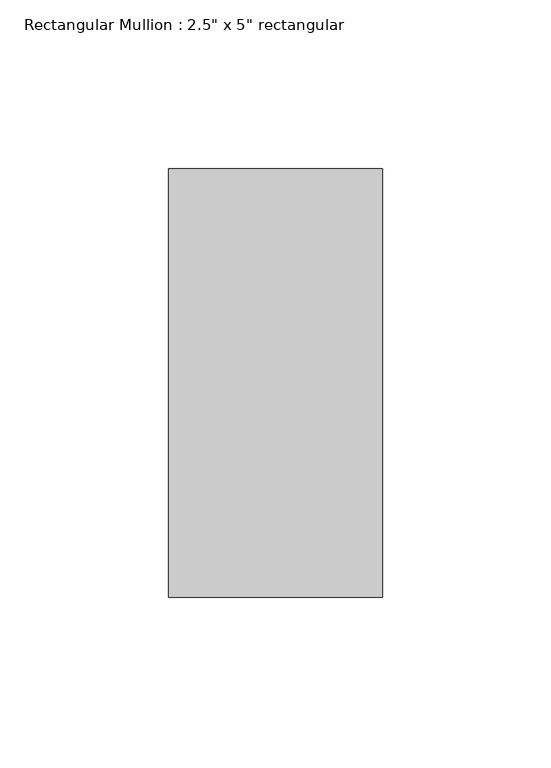
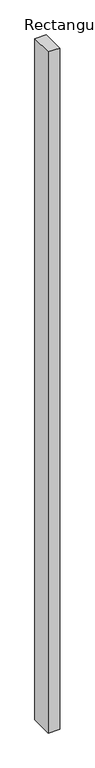
"""IFC4 building model written with IfcOpenShell, lengths in millimetres: member geometry."""

from ifc_helpers import new_model, si_unit, frame, origin, place, context, project, spatial, polyline, outline, extrude, source, transform, mapped, element, save


def member_3472e6fb(model_context):
    return source(origin(), model_context, "Body", "SweptSolid", [
        extrude(outline(polyline([(0.0, 63.5), (0.0, -63.5), (-63.5, -63.5), (-63.5, 63.5), (0.0, 63.5)])), frame((0.0, 0.0, -3960.0609328), z_axis=(0.0, 0.0, 1.0), x_axis=(1.0, 0.0, 0.0)), (0.0, 0.0, 1.0), 3960.0609328),
    ])


if __name__ == "__main__":
    model = new_model("IFC4")
    model_context = context("Model", 3, world=origin())
    ifc_project = project(units=[si_unit("LENGTHUNIT", "METRE", prefix="MILLI")], contexts=[model_context])
    site = spatial("IfcSite", under=ifc_project)
    building = spatial("IfcBuilding", under=site)
    placement = place(None, origin())
    member_shape = member_3472e6fb(model_context)
    element("IfcMember", 1, ObjectType="Rectangular Mullion : 2.5\" x 5\" rectangular", at=placement, inside=building, context=model_context, shape_type="MappedRepresentation", body=[
        mapped(member_shape, transform((0.0, 0.0, 0.0), x_axis=(1.0, 0.0, 0.0), y_axis=(0.0, 1.0, 0.0), z_axis=(0.0, 0.0, 1.0))),
    ])
    save(model, "model.ifc")

# Revit data of these elements
# Type "Rectangular Mullion : 2.5\" x 5\" rectangular"
#   built-in parameter 1007304 = 0.416667 (stored number, unit not read)
#   built-in parameter 1007301 = 0.104167 (stored number, unit not read)
#   built-in parameter 1007300 = 0.104167 (stored number, unit not read)
# Element 1 (IfcMember, "Rectangular Mullion : 2.5\" x 5\" rectangular")
#   Materials on its faces: "Aluminum"
# Materials
#   "Aluminum": class "Metal", colour RGB 247 247 247, transparency 0, Description = "Aluminum 6061", Cost = 0
